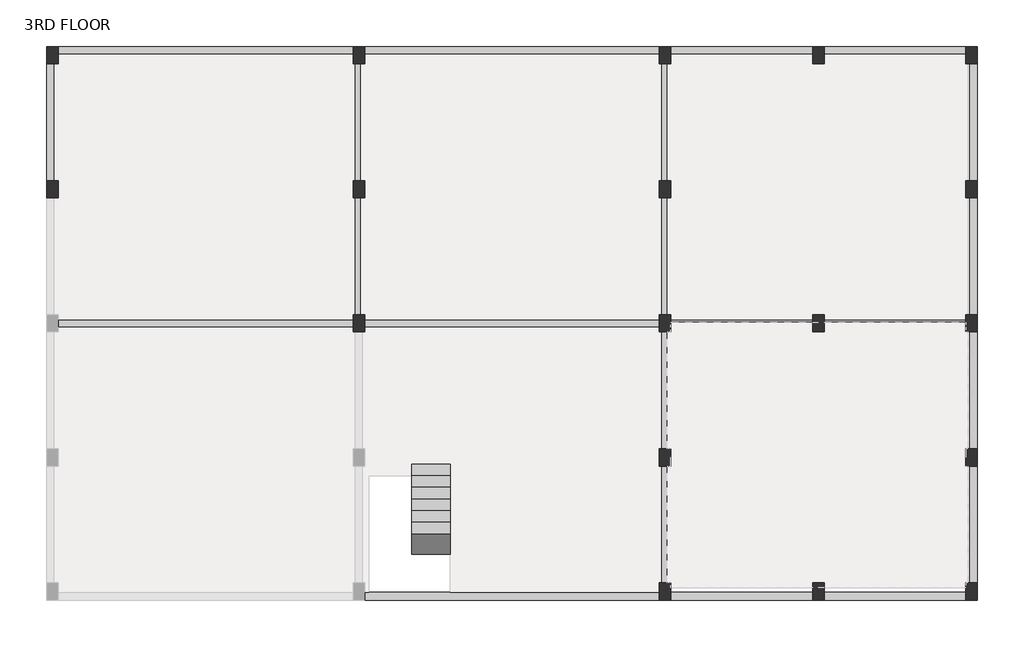
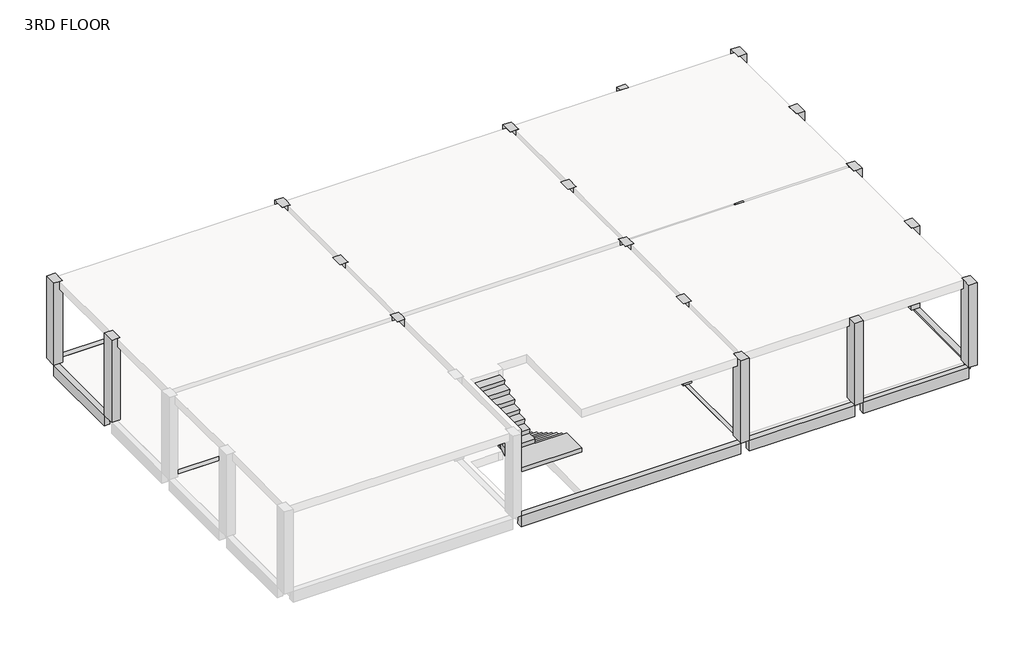
# One storey, part 2 of 2: 22 beams, 18 columns, 1 stair flight.
"""IFC4 building model written with IfcOpenShell, lengths in millimetres."""

from ifc_helpers import new_model, si_unit, frame, origin, place, context, project, spatial, polyline, outline, extrude, faceted_brep, element, save

model = new_model("IFC4")

# Units and contexts
model_context = context("Model", 3, world=origin())
ifc_project = project(units=[si_unit("LENGTHUNIT", "METRE", prefix="MILLI")], contexts=[model_context])

# Site, building, storey
site = spatial("IfcSite", under=ifc_project)
building = spatial("IfcBuilding", under=site)
storey = spatial("IfcBuildingStorey", under=building, Name="3RD FLOOR", Elevation=9144.0)

# Beams
placement = place(None, origin())
element("IfcBeam", 1, ObjectType="M_Concrete-Rectangular Beam : 200MMX400MM", at=placement, inside=storey, context=model_context, shape_type="Brep", body=[
    faceted_brep([(-3980.6874017, 15797.7008557, 9144.0), (-3980.6874017, 15997.7008557, 9144.0), (-11680.6874017, 15997.7008557, 9144.0), (-11680.6874017, 15797.7008557, 9144.0), (-3980.6874017, 15797.7008557, 8744.0), (-3980.6874017, 15797.7008557, 8844.0), (-11680.6874017, 15797.7008557, 8844.0), (-11680.6874017, 15797.7008557, 8744.0), (-3980.6874017, 15997.7008557, 8744.0), (-11680.6874017, 15997.7008557, 8744.0)], [[[0, 1, 2, 3]], [[4, 5, 0, 3, 6, 7]], [[8, 4, 7, 9]], [[1, 8, 9, 2]], [[2, 9, 7, 6, 3]], [[1, 0, 5, 4, 8]]]),
])
element("IfcBeam", 2, ObjectType="M_Concrete-Rectangular Beam : 200MMX400MM", at=placement, inside=storey, context=model_context, shape_type="Brep", body=[
    faceted_brep([(4019.3125983, 15797.7008557, 9144.0), (4019.3125983, 15997.7008557, 9144.0), (-3680.6874017, 15997.7008557, 9144.0), (-3680.6874017, 15797.7008557, 9144.0), (4019.3125983, 15797.7008557, 8744.0), (4019.3125983, 15797.7008557, 8844.0), (-3680.6874017, 15797.7008557, 8844.0), (-3680.6874017, 15797.7008557, 8744.0), (4019.3125983, 15997.7008557, 8744.0), (-3680.6874017, 15997.7008557, 8744.0)], [[[0, 1, 2, 3]], [[4, 5, 0, 3, 6, 7]], [[8, 4, 7, 9]], [[1, 8, 9, 2]], [[1, 0, 5, 4, 8]], [[2, 9, 7, 6, 3]]]),
])
element("IfcBeam", 3, ObjectType="M_Concrete-Rectangular Beam : 200MMX400MM", at=placement, inside=storey, context=model_context, shape_type="Brep", body=[
    faceted_brep([(8019.3125983, 15797.7008557, 9144.0), (8019.3125983, 15997.7008557, 9144.0), (4319.3125983, 15997.7008557, 9144.0), (4319.3125983, 15797.7008557, 9144.0), (8019.3125983, 15797.7008557, 8744.0), (4319.3125983, 15797.7008557, 8844.0), (4319.3125983, 15797.7008557, 8744.0), (8019.3125983, 15997.7008557, 8744.0), (4319.3125983, 15997.7008557, 8744.0)], [[[0, 1, 2, 3]], [[4, 0, 3, 5, 6]], [[7, 4, 6, 8]], [[1, 7, 8, 2]], [[2, 8, 6, 5, 3]], [[1, 0, 4, 7]]]),
])
element("IfcBeam", 4, ObjectType="M_Concrete-Rectangular Beam : 200MMX400MM", at=placement, inside=storey, context=model_context, shape_type="Brep", body=[
    faceted_brep([(12019.3125983, 15797.7008557, 9144.0), (12019.3125983, 15997.7008557, 9144.0), (8319.3125983, 15997.7008557, 9144.0), (8319.3125983, 15797.7008557, 9144.0), (12019.3125983, 15797.7008557, 8744.0), (12019.3125983, 15797.7008557, 8844.0), (8319.3125983, 15797.7008557, 8744.0), (12019.3125983, 15997.7008557, 8744.0), (8319.3125983, 15997.7008557, 8744.0)], [[[0, 1, 2, 3]], [[4, 5, 0, 3, 6]], [[7, 4, 6, 8]], [[1, 7, 8, 2]], [[2, 8, 6, 3]], [[1, 0, 5, 4, 7]]]),
])
element("IfcBeam", 5, ObjectType="M_Concrete-Rectangular Beam : 200MMX400MM", at=placement, inside=storey, context=model_context, shape_type="SweptSolid", body=[
    extrude(outline(polyline([(12319.3125983, 12497.7008557), (12119.3125983, 12497.7008557), (12119.3125983, 15547.7008557), (12319.3125983, 15547.7008557), (12319.3125983, 12497.7008557)])), frame((0.0, 0.0, 8744.0), z_axis=(0.0, 0.0, 1.0), x_axis=(1.0, 0.0, 0.0)), (0.0, 0.0, 1.0), 400.0),
])
element("IfcBeam", 6, ObjectType="M_Concrete-Rectangular Beam : 200MMX400MM", at=placement, inside=storey, context=model_context, shape_type="SweptSolid", body=[
    extrude(outline(polyline([(12319.3125983, 1997.7008557), (12119.3125983, 1997.7008557), (12119.3125983, 5047.7008557), (12319.3125983, 5047.7008557), (12319.3125983, 1997.7008557)])), frame((0.0, 0.0, 8744.0), z_axis=(0.0, 0.0, 1.0), x_axis=(1.0, 0.0, 0.0)), (0.0, 0.0, 1.0), 400.0),
])
element("IfcBeam", 7, ObjectType="M_Concrete-Rectangular Beam : 200MMX400MM", at=placement, inside=storey, context=model_context, shape_type="SweptSolid", body=[
    extrude(outline(polyline([(8319.3125983, 1547.7008557), (8319.3125983, 1747.7008557), (12019.3125983, 1747.7008557), (12019.3125983, 1547.7008557), (8319.3125983, 1547.7008557)])), frame((0.0, 0.0, 8744.0), z_axis=(0.0, 0.0, 1.0), x_axis=(1.0, 0.0, 0.0)), (0.0, 0.0, 1.0), 400.0),
])
element("IfcBeam", 8, ObjectType="M_Concrete-Rectangular Beam : 200MMX400MM", at=placement, inside=storey, context=model_context, shape_type="SweptSolid", body=[
    extrude(outline(polyline([(8019.3125983, 1747.7008557), (8019.3125983, 1547.7008557), (4319.3125983, 1547.7008557), (4319.3125983, 1747.7008557), (8019.3125983, 1747.7008557)])), frame((0.0, 0.0, 8744.0), z_axis=(0.0, 0.0, 1.0), x_axis=(1.0, 0.0, 0.0)), (0.0, 0.0, 1.0), 400.0),
])
element("IfcBeam", 9, ObjectType="M_Concrete-Rectangular Beam : 200MMX400MM", at=placement, inside=storey, context=model_context, shape_type="Brep", body=[
    faceted_brep([(-3680.6874017, 1747.7008557, 9144.0), (-3680.6874017, 1547.7008557, 9144.0), (4019.3125983, 1547.7008557, 9144.0), (4019.3125983, 1747.7008557, 9144.0), (-1437.0874017, 1747.7008557, 9144.0), (-3570.6874017, 1747.7008557, 9144.0), (-3680.6874017, 1747.7008557, 8744.0), (-3680.6874017, 1747.7008557, 8844.0), (4019.3125983, 1747.7008557, 8844.0), (4019.3125983, 1747.7008557, 8744.0), (-3680.6874017, 1547.7008557, 8744.0), (4019.3125983, 1547.7008557, 8744.0)], [[[0, 1, 2, 3, 4, 5]], [[6, 7, 0, 5, 4, 3, 8, 9]], [[10, 6, 9, 11]], [[1, 10, 11, 2]], [[1, 0, 7, 6, 10]], [[2, 11, 9, 8, 3]]]),
])
element("IfcBeam", 10, ObjectType="M_Concrete-Rectangular Beam : 200MMX400MM", at=placement, inside=storey, context=model_context, shape_type="Brep", body=[
    faceted_brep([(-3980.6874017, 8872.7008557, 9144.0), (-11680.6874017, 8872.7008557, 9144.0), (-11680.6874017, 8672.7008557, 9144.0), (-3980.6874017, 8672.7008557, 9144.0), (-11680.6874017, 8672.7008557, 8844.0), (-11680.6874017, 8672.7008557, 8744.0), (-3980.6874017, 8672.7008557, 8744.0), (-3980.6874017, 8672.7008557, 8844.0), (-11680.6874017, 8872.7008557, 8744.0), (-3980.6874017, 8872.7008557, 8744.0), (-3980.6874017, 8872.7008557, 8844.0), (-11680.6874017, 8872.7008557, 8844.0)], [[[0, 1, 2, 3]], [[3, 2, 4, 5, 6, 7]], [[6, 5, 8, 9]], [[1, 0, 10, 9, 8, 11]], [[8, 5, 4, 2, 1, 11]], [[0, 3, 7, 6, 9, 10]]]),
])
element("IfcBeam", 11, ObjectType="M_Concrete-Rectangular Beam : 200MMX400MM", at=placement, inside=storey, context=model_context, shape_type="Brep", body=[
    faceted_brep([(4019.3125983, 8872.7008557, 9144.0), (-3680.6874017, 8872.7008557, 9144.0), (-3680.6874017, 8672.7008557, 9144.0), (4019.3125983, 8672.7008557, 9144.0), (-3680.6874017, 8672.7008557, 8844.0), (-3680.6874017, 8672.7008557, 8744.0), (4019.3125983, 8672.7008557, 8744.0), (4019.3125983, 8672.7008557, 8844.0), (-3680.6874017, 8872.7008557, 8744.0), (4019.3125983, 8872.7008557, 8744.0), (4019.3125983, 8872.7008557, 8844.0), (-3680.6874017, 8872.7008557, 8844.0)], [[[0, 1, 2, 3]], [[3, 2, 4, 5, 6, 7]], [[6, 5, 8, 9]], [[1, 0, 10, 9, 8, 11]], [[8, 5, 4, 2, 1, 11]], [[0, 3, 7, 6, 9, 10]]]),
])
element("IfcBeam", 12, ObjectType="M_Concrete-Rectangular Beam : 200MMX400MM", at=placement, inside=storey, context=model_context, shape_type="Brep", body=[
    faceted_brep([(8019.3125983, 8872.7008557, 9144.0), (4319.3125983, 8872.7008557, 9144.0), (4319.3125983, 8797.7008557, 9144.0), (8019.3125983, 8797.7008557, 9144.0), (4319.3125983, 8672.7008557, 8744.0), (8019.3125983, 8672.7008557, 8744.0), (8019.3125983, 8672.7008557, 8844.0), (4319.3125983, 8672.7008557, 8844.0), (4319.3125983, 8872.7008557, 8744.0), (8019.3125983, 8872.7008557, 8744.0), (8019.3125983, 8872.7008557, 8844.0), (4319.3125983, 8872.7008557, 8844.0), (4319.3125983, 8797.7008557, 8844.0), (8019.3125983, 8797.7008557, 8844.0)], [[[0, 1, 2, 3]], [[4, 5, 6, 7]], [[5, 4, 8, 9]], [[1, 0, 10, 9, 8, 11]], [[8, 4, 7, 12, 2, 1, 11]], [[5, 9, 10, 0, 3, 13, 6]], [[13, 12, 7, 6]], [[12, 13, 3, 2]]]),
])
element("IfcBeam", 13, ObjectType="M_Concrete-Rectangular Beam : 200MMX400MM", at=placement, inside=storey, context=model_context, shape_type="Brep", body=[
    faceted_brep([(-11980.6874017, 12497.7008557, 9144.0), (-11780.6874017, 12497.7008557, 9144.0), (-11780.6874017, 15547.7008557, 9144.0), (-11980.6874017, 15547.7008557, 9144.0), (-11980.6874017, 12497.7008557, 8744.0), (-11980.6874017, 15547.7008557, 8744.0), (-11780.6874017, 12497.7008557, 8744.0), (-11780.6874017, 15547.7008557, 8744.0), (-11780.6874017, 12497.7008557, 8844.0), (-11780.6874017, 15547.7008557, 8844.0)], [[[0, 1, 2, 3]], [[4, 0, 3, 5]], [[6, 4, 5, 7]], [[1, 8, 6, 7, 9, 2]], [[2, 9, 7, 5, 3]], [[1, 0, 4, 6, 8]]]),
])
element("IfcBeam", 14, ObjectType="M_Concrete-Rectangular Beam : 200MMX400MM", at=placement, inside=storey, context=model_context, shape_type="Brep", body=[
    faceted_brep([(12019.3125983, 8872.7008557, 9144.0), (8319.3125983, 8872.7008557, 9144.0), (8319.3125983, 8797.7008557, 9144.0), (12019.3125983, 8797.7008557, 9144.0), (8319.3125983, 8672.7008557, 8744.0), (12019.3125983, 8672.7008557, 8744.0), (12019.3125983, 8672.7008557, 8844.0), (8319.3125983, 8672.7008557, 8844.0), (8319.3125983, 8872.7008557, 8744.0), (12019.3125983, 8872.7008557, 8744.0), (12019.3125983, 8872.7008557, 8844.0), (8319.3125983, 8872.7008557, 8844.0), (12019.3125983, 8797.7008557, 8844.0), (8319.3125983, 8797.7008557, 8844.0)], [[[0, 1, 2, 3]], [[4, 5, 6, 7]], [[5, 4, 8, 9]], [[1, 0, 10, 9, 8, 11]], [[5, 9, 10, 0, 3, 12, 6]], [[8, 4, 7, 13, 2, 1, 11]], [[12, 13, 7, 6]], [[13, 12, 3, 2]]]),
])
element("IfcBeam", 15, ObjectType="M_Concrete-Rectangular Beam : 200MMX400MM", at=placement, inside=storey, context=model_context, shape_type="SweptSolid", body=[
    extrude(outline(polyline([(12319.3125983, 5497.7008557), (12119.3125983, 5497.7008557), (12119.3125983, 8547.7008557), (12319.3125983, 8547.7008557), (12319.3125983, 5497.7008557)])), frame((0.0, 0.0, 8744.0), z_axis=(0.0, 0.0, 1.0), x_axis=(1.0, 0.0, 0.0)), (0.0, 0.0, 1.0), 400.0),
])
element("IfcBeam", 16, ObjectType="M_Concrete-Rectangular Beam : 200MMX400MM", at=placement, inside=storey, context=model_context, shape_type="SweptSolid", body=[
    extrude(outline(polyline([(12119.3125983, 12047.7008557), (12319.3125983, 12047.7008557), (12319.3125983, 8997.7008557), (12119.3125983, 8997.7008557), (12119.3125983, 12047.7008557)])), frame((0.0, 0.0, 8744.0), z_axis=(0.0, 0.0, 1.0), x_axis=(1.0, 0.0, 0.0)), (0.0, 0.0, 1.0), 400.0),
])
element("IfcBeam", 17, ObjectType="M_Concrete-Rectangular Beam : 200MMX400MM", at=placement, inside=storey, context=model_context, shape_type="Brep", body=[
    faceted_brep([(4069.3125983, 5047.7008557, 9144.0), (4069.3125983, 1997.7008557, 9144.0), (4219.3125983, 1997.7008557, 9144.0), (4219.3125983, 5047.7008557, 9144.0), (4269.3125983, 1997.7008557, 8744.0), (4269.3125983, 5047.7008557, 8744.0), (4269.3125983, 5047.7008557, 8844.0), (4269.3125983, 1997.7008557, 8844.0), (4069.3125983, 1997.7008557, 8744.0), (4069.3125983, 5047.7008557, 8744.0), (4069.3125983, 5047.7008557, 8844.0), (4069.3125983, 1997.7008557, 8844.0), (4219.3125983, 1997.7008557, 8844.0), (4219.3125983, 5047.7008557, 8844.0)], [[[0, 1, 2, 3]], [[4, 5, 6, 7]], [[5, 4, 8, 9]], [[1, 0, 10, 9, 8, 11]], [[8, 4, 7, 12, 2, 1, 11]], [[5, 9, 10, 0, 3, 13, 6]], [[13, 12, 7, 6]], [[12, 13, 3, 2]]]),
])
element("IfcBeam", 18, ObjectType="M_Concrete-Rectangular Beam : 200MMX400MM", at=placement, inside=storey, context=model_context, shape_type="Brep", body=[
    faceted_brep([(4069.3125983, 8547.7008557, 9144.0), (4069.3125983, 5497.7008557, 9144.0), (4219.3125983, 5497.7008557, 9144.0), (4219.3125983, 8547.7008557, 9144.0), (4269.3125983, 5497.7008557, 8744.0), (4269.3125983, 8547.7008557, 8744.0), (4269.3125983, 8547.7008557, 8844.0), (4269.3125983, 5497.7008557, 8844.0), (4069.3125983, 5497.7008557, 8744.0), (4069.3125983, 8547.7008557, 8744.0), (4069.3125983, 8547.7008557, 8844.0), (4069.3125983, 5497.7008557, 8844.0), (4219.3125983, 8547.7008557, 8844.0), (4219.3125983, 5497.7008557, 8844.0)], [[[0, 1, 2, 3]], [[4, 5, 6, 7]], [[5, 4, 8, 9]], [[1, 0, 10, 9, 8, 11]], [[5, 9, 10, 0, 3, 12, 6]], [[8, 4, 7, 13, 2, 1, 11]], [[12, 13, 7, 6]], [[13, 12, 3, 2]]]),
])
element("IfcBeam", 19, ObjectType="M_Concrete-Rectangular Beam : 200MMX400MM", at=placement, inside=storey, context=model_context, shape_type="Brep", body=[
    faceted_brep([(4069.3125983, 12047.7008557, 9144.0), (4069.3125983, 8997.7008557, 9144.0), (4219.3125983, 8997.7008557, 9144.0), (4219.3125983, 12047.7008557, 9144.0), (4269.3125983, 8997.7008557, 8744.0), (4269.3125983, 12047.7008557, 8744.0), (4269.3125983, 12047.7008557, 8844.0), (4269.3125983, 8997.7008557, 8844.0), (4069.3125983, 8997.7008557, 8744.0), (4069.3125983, 12047.7008557, 8744.0), (4069.3125983, 12047.7008557, 8844.0), (4069.3125983, 8997.7008557, 8844.0), (4219.3125983, 8997.7008557, 8844.0), (4219.3125983, 12047.7008557, 8844.0)], [[[0, 1, 2, 3]], [[4, 5, 6, 7]], [[5, 4, 8, 9]], [[1, 0, 10, 9, 8, 11]], [[8, 4, 7, 12, 2, 1, 11]], [[5, 9, 10, 0, 3, 13, 6]], [[13, 12, 7, 6]], [[12, 13, 3, 2]]]),
])
element("IfcBeam", 20, ObjectType="M_Concrete-Rectangular Beam : 200MMX400MM", at=placement, inside=storey, context=model_context, shape_type="Brep", body=[
    faceted_brep([(4069.3125983, 15547.7008557, 9144.0), (4069.3125983, 12497.7008557, 9144.0), (4219.3125983, 12497.7008557, 9144.0), (4219.3125983, 15547.7008557, 9144.0), (4269.3125983, 12497.7008557, 8744.0), (4269.3125983, 15547.7008557, 8744.0), (4269.3125983, 15547.7008557, 8844.0), (4269.3125983, 12497.7008557, 8844.0), (4069.3125983, 12497.7008557, 8744.0), (4069.3125983, 15547.7008557, 8744.0), (4069.3125983, 15547.7008557, 8844.0), (4069.3125983, 12497.7008557, 8844.0), (4219.3125983, 15547.7008557, 8844.0), (4219.3125983, 12497.7008557, 8844.0)], [[[0, 1, 2, 3]], [[4, 5, 6, 7]], [[5, 4, 8, 9]], [[1, 0, 10, 9, 8, 11]], [[5, 9, 10, 0, 3, 12, 6]], [[8, 4, 7, 13, 2, 1, 11]], [[12, 13, 7, 6]], [[13, 12, 3, 2]]]),
])
element("IfcBeam", 21, ObjectType="M_Concrete-Rectangular Beam : 200MMX400MM", at=placement, inside=storey, context=model_context, shape_type="Brep", body=[
    faceted_brep([(-3930.6874017, 12047.7008557, 9144.0), (-3930.6874017, 8997.7008557, 9144.0), (-3780.6874017, 8997.7008557, 9144.0), (-3780.6874017, 12047.7008557, 9144.0), (-3730.6874017, 8997.7008557, 8744.0), (-3730.6874017, 12047.7008557, 8744.0), (-3730.6874017, 12047.7008557, 8844.0), (-3730.6874017, 8997.7008557, 8844.0), (-3930.6874017, 8997.7008557, 8744.0), (-3930.6874017, 12047.7008557, 8744.0), (-3930.6874017, 12047.7008557, 8844.0), (-3930.6874017, 8997.7008557, 8844.0), (-3780.6874017, 12047.7008557, 8844.0), (-3780.6874017, 8997.7008557, 8844.0)], [[[0, 1, 2, 3]], [[4, 5, 6, 7]], [[5, 4, 8, 9]], [[1, 0, 10, 9, 8, 11]], [[5, 9, 10, 0, 3, 12, 6]], [[8, 4, 7, 13, 2, 1, 11]], [[12, 13, 7, 6]], [[13, 12, 3, 2]]]),
])
element("IfcBeam", 22, ObjectType="M_Concrete-Rectangular Beam : 200MMX400MM", at=placement, inside=storey, context=model_context, shape_type="Brep", body=[
    faceted_brep([(-3930.6874017, 15547.7008557, 9144.0), (-3930.6874017, 12497.7008557, 9144.0), (-3780.6874017, 12497.7008557, 9144.0), (-3780.6874017, 15547.7008557, 9144.0), (-3730.6874017, 12497.7008557, 8744.0), (-3730.6874017, 15547.7008557, 8744.0), (-3730.6874017, 15547.7008557, 8844.0), (-3730.6874017, 12497.7008557, 8844.0), (-3930.6874017, 12497.7008557, 8744.0), (-3930.6874017, 15547.7008557, 8744.0), (-3930.6874017, 15547.7008557, 8844.0), (-3930.6874017, 12497.7008557, 8844.0), (-3780.6874017, 15547.7008557, 8844.0), (-3780.6874017, 12497.7008557, 8844.0)], [[[0, 1, 2, 3]], [[4, 5, 6, 7]], [[5, 4, 8, 9]], [[1, 0, 10, 9, 8, 11]], [[5, 9, 10, 0, 3, 12, 6]], [[8, 4, 7, 13, 2, 1, 11]], [[12, 13, 7, 6]], [[13, 12, 3, 2]]]),
])

# Columns
element("IfcColumn", 23, ObjectType="M_Concrete-Rectangular-Column : 300 x 450mm", at=placement, inside=storey, context=model_context, shape_type="Brep", body=[
    faceted_brep([(-11680.6874017, 15997.7008557, 9144.0), (-11680.6874017, 15547.7008557, 9144.0), (-11980.6874017, 15547.7008557, 9144.0), (-11980.6874017, 15997.7008557, 9144.0), (-11680.6874017, 15997.7008557, 12192.0), (-11680.6874017, 15797.7008557, 12192.0), (-11680.6874017, 15547.7008557, 12192.0), (-11680.6874017, 15547.7008557, 11892.0), (-11780.6874017, 15547.7008557, 12192.0), (-11980.6874017, 15547.7008557, 12192.0), (-11980.6874017, 15997.7008557, 12192.0)], [[[0, 1, 2, 3]], [[1, 0, 4, 5, 6, 7]], [[2, 1, 7, 6, 8, 9]], [[3, 2, 9, 10]], [[0, 3, 10, 4]], [[10, 9, 8, 6, 5, 4]]]),
])
element("IfcColumn", 24, ObjectType="M_Concrete-Rectangular-Column : 300 x 450mm", at=placement, inside=storey, context=model_context, shape_type="Brep", body=[
    faceted_brep([(-3680.6874017, 15997.7008557, 9144.0), (-3680.6874017, 15547.7008557, 9144.0), (-3980.6874017, 15547.7008557, 9144.0), (-3980.6874017, 15997.7008557, 9144.0), (-3680.6874017, 15997.7008557, 12192.0), (-3680.6874017, 15797.7008557, 12192.0), (-3680.6874017, 15547.7008557, 12192.0), (-3680.6874017, 15547.7008557, 11892.0), (-3780.6874017, 15547.7008557, 12192.0), (-3930.6874017, 15547.7008557, 12192.0), (-3980.6874017, 15547.7008557, 12192.0), (-3980.6874017, 15547.7008557, 11892.0), (-3980.6874017, 15797.7008557, 12192.0), (-3980.6874017, 15997.7008557, 12192.0)], [[[0, 1, 2, 3]], [[1, 0, 4, 5, 6, 7]], [[2, 1, 7, 6, 8, 9, 10, 11]], [[3, 2, 11, 10, 12, 13]], [[0, 3, 13, 4]], [[4, 13, 12, 10, 9, 8, 6, 5]]]),
])
element("IfcColumn", 25, ObjectType="M_Concrete-Rectangular-Column : 300 x 450mm", at=placement, inside=storey, context=model_context, shape_type="Brep", body=[
    faceted_brep([(-3680.6874017, 12497.7008557, 9144.0), (-3680.6874017, 12047.7008557, 9144.0), (-3980.6874017, 12047.7008557, 9144.0), (-3980.6874017, 12497.7008557, 9144.0), (-3680.6874017, 12497.7008557, 11892.0), (-3680.6874017, 12497.7008557, 12192.0), (-3680.6874017, 12047.7008557, 12192.0), (-3680.6874017, 12047.7008557, 11892.0), (-3780.6874017, 12047.7008557, 12192.0), (-3930.6874017, 12047.7008557, 12192.0), (-3980.6874017, 12047.7008557, 12192.0), (-3980.6874017, 12047.7008557, 11892.0), (-3980.6874017, 12497.7008557, 12192.0), (-3980.6874017, 12497.7008557, 11892.0), (-3930.6874017, 12497.7008557, 12192.0), (-3780.6874017, 12497.7008557, 12192.0)], [[[0, 1, 2, 3]], [[1, 0, 4, 5, 6, 7]], [[2, 1, 7, 6, 8, 9, 10, 11]], [[3, 2, 11, 10, 12, 13]], [[0, 3, 13, 12, 14, 15, 5, 4]], [[6, 5, 15, 14, 12, 10, 9, 8]]]),
])
element("IfcColumn", 26, ObjectType="M_Concrete-Rectangular-Column : 300 x 450mm", at=placement, inside=storey, context=model_context, shape_type="Brep", body=[
    faceted_brep([(-3680.6874017, 8997.7008557, 9144.0), (-3680.6874017, 8547.7008557, 9144.0), (-3980.6874017, 8547.7008557, 9144.0), (-3980.6874017, 8997.7008557, 9144.0), (-3680.6874017, 8997.7008557, 11892.0), (-3680.6874017, 8997.7008557, 12192.0), (-3680.6874017, 8872.7008557, 12192.0), (-3680.6874017, 8672.7008557, 12192.0), (-3680.6874017, 8547.7008557, 12192.0), (-3680.6874017, 8547.7008557, 11892.0), (-3730.6874017, 8547.7008557, 12192.0), (-3930.6874017, 8547.7008557, 12192.0), (-3980.6874017, 8547.7008557, 12192.0), (-3980.6874017, 8547.7008557, 11892.0), (-3980.6874017, 8672.7008557, 12192.0), (-3980.6874017, 8872.7008557, 12192.0), (-3980.6874017, 8997.7008557, 12192.0), (-3980.6874017, 8997.7008557, 11892.0), (-3930.6874017, 8997.7008557, 12192.0), (-3780.6874017, 8997.7008557, 12192.0)], [[[0, 1, 2, 3]], [[1, 0, 4, 5, 6, 7, 8, 9]], [[2, 1, 9, 8, 10, 11, 12, 13]], [[3, 2, 13, 12, 14, 15, 16, 17]], [[0, 3, 17, 16, 18, 19, 5, 4]], [[18, 16, 15, 14, 12, 11, 10, 8, 7, 6, 5, 19]]]),
])
element("IfcColumn", 27, ObjectType="M_Concrete-Rectangular-Column : 300 x 450mm", at=placement, inside=storey, context=model_context, shape_type="Brep", body=[
    faceted_brep([(4319.3125983, 15997.7008557, 9144.0), (4319.3125983, 15547.7008557, 9144.0), (4019.3125983, 15547.7008557, 9144.0), (4019.3125983, 15997.7008557, 9144.0), (4319.3125983, 15997.7008557, 12192.0), (4319.3125983, 15797.7008557, 12192.0), (4319.3125983, 15547.7008557, 12192.0), (4319.3125983, 15547.7008557, 11892.0), (4219.3125983, 15547.7008557, 12192.0), (4069.3125983, 15547.7008557, 12192.0), (4019.3125983, 15547.7008557, 12192.0), (4019.3125983, 15547.7008557, 11892.0), (4019.3125983, 15797.7008557, 12192.0), (4019.3125983, 15997.7008557, 12192.0)], [[[0, 1, 2, 3]], [[1, 0, 4, 5, 6, 7]], [[2, 1, 7, 6, 8, 9, 10, 11]], [[3, 2, 11, 10, 12, 13]], [[0, 3, 13, 4]], [[4, 13, 12, 10, 9, 8, 6, 5]]]),
])
element("IfcColumn", 28, ObjectType="M_Concrete-Rectangular-Column : 300 x 450mm", at=placement, inside=storey, context=model_context, shape_type="Brep", body=[
    faceted_brep([(4319.3125983, 8997.7008557, 9144.0), (4319.3125983, 8547.7008557, 9144.0), (4019.3125983, 8547.7008557, 9144.0), (4019.3125983, 8997.7008557, 9144.0), (4319.3125983, 8997.7008557, 11892.0), (4319.3125983, 8997.7008557, 12192.0), (4319.3125983, 8872.7008557, 12192.0), (4319.3125983, 8797.7008557, 12192.0), (4319.3125983, 8547.7008557, 12192.0), (4319.3125983, 8547.7008557, 11892.0), (4219.3125983, 8547.7008557, 12192.0), (4069.3125983, 8547.7008557, 12192.0), (4019.3125983, 8547.7008557, 12192.0), (4019.3125983, 8547.7008557, 11892.0), (4019.3125983, 8672.7008557, 12192.0), (4019.3125983, 8872.7008557, 12192.0), (4019.3125983, 8997.7008557, 12192.0), (4019.3125983, 8997.7008557, 11892.0), (4069.3125983, 8997.7008557, 12192.0), (4219.3125983, 8997.7008557, 12192.0)], [[[0, 1, 2, 3]], [[1, 0, 4, 5, 6, 7, 8, 9]], [[2, 1, 9, 8, 10, 11, 12, 13]], [[3, 2, 13, 12, 14, 15, 16, 17]], [[0, 3, 17, 16, 18, 19, 5, 4]], [[18, 16, 15, 14, 12, 11, 10, 8, 7, 6, 5, 19]]]),
])
element("IfcColumn", 29, ObjectType="M_Concrete-Rectangular-Column : 300 x 450mm", at=placement, inside=storey, context=model_context, shape_type="Brep", body=[
    faceted_brep([(4319.3125983, 1997.7008557, 9144.0), (4319.3125983, 1547.7008557, 9144.0), (4019.3125983, 1547.7008557, 9144.0), (4019.3125983, 1997.7008557, 9144.0), (4319.3125983, 1997.7008557, 11892.0), (4319.3125983, 1997.7008557, 12192.0), (4319.3125983, 1872.7008557, 12192.0), (4319.3125983, 1547.7008557, 12192.0), (4019.3125983, 1547.7008557, 12192.0), (4019.3125983, 1747.7008557, 12192.0), (4019.3125983, 1997.7008557, 12192.0), (4019.3125983, 1997.7008557, 11892.0), (4069.3125983, 1997.7008557, 12192.0), (4219.3125983, 1997.7008557, 12192.0)], [[[0, 1, 2, 3]], [[1, 0, 4, 5, 6, 7]], [[2, 1, 7, 8]], [[3, 2, 8, 9, 10, 11]], [[0, 3, 11, 10, 12, 13, 5, 4]], [[8, 7, 6, 5, 13, 12, 10, 9]]]),
])
element("IfcColumn", 30, ObjectType="M_Concrete-Rectangular-Column : 300 x 450mm", at=placement, inside=storey, context=model_context, shape_type="SweptSolid", body=[
    extrude(outline(polyline([(15997.7008557, 9144.0), (15547.7008557, 9144.0), (15547.7008557, 11892.0), (15797.7008557, 11892.0), (15797.7008557, 12192.0), (15997.7008557, 12192.0), (15997.7008557, 9144.0)])), frame((8019.3125983, 0.0, 0.0), z_axis=(1.0, 0.0, 0.0), x_axis=(0.0, 1.0, 0.0)), (0.0, 0.0, 1.0), 300.0),
])
element("IfcColumn", 31, ObjectType="M_Concrete-Rectangular-Column : 300 x 450mm", at=placement, inside=storey, context=model_context, shape_type="SweptSolid", body=[
    extrude(outline(polyline([(1997.7008557, 9144.0), (1547.7008557, 9144.0), (1547.7008557, 12192.0), (1872.7008557, 12192.0), (1872.7008557, 11892.0), (1997.7008557, 11892.0), (1997.7008557, 9144.0)])), frame((8019.3125983, 0.0, 0.0), z_axis=(1.0, 0.0, 0.0), x_axis=(0.0, 1.0, 0.0)), (0.0, 0.0, 1.0), 300.0),
])
element("IfcColumn", 32, ObjectType="M_Concrete-Rectangular-Column : 300 x 450mm", at=placement, inside=storey, context=model_context, shape_type="Brep", body=[
    faceted_brep([(12319.3125983, 12497.7008557, 9144.0), (12319.3125983, 12047.7008557, 9144.0), (12019.3125983, 12047.7008557, 9144.0), (12019.3125983, 12497.7008557, 9144.0), (12319.3125983, 12497.7008557, 12192.0), (12319.3125983, 12047.7008557, 12192.0), (12069.3125983, 12047.7008557, 12192.0), (12019.3125983, 12047.7008557, 12192.0), (12019.3125983, 12047.7008557, 11892.0), (12019.3125983, 12497.7008557, 12192.0), (12019.3125983, 12497.7008557, 11892.0), (12069.3125983, 12497.7008557, 12192.0)], [[[0, 1, 2, 3]], [[1, 0, 4, 5]], [[2, 1, 5, 6, 7, 8]], [[3, 2, 8, 7, 9, 10]], [[0, 3, 10, 9, 11, 4]], [[5, 4, 11, 9, 7, 6]]]),
])
element("IfcColumn", 33, ObjectType="M_Concrete-Rectangular-Column : 300 x 450mm", at=placement, inside=storey, context=model_context, shape_type="Brep", body=[
    faceted_brep([(12319.3125983, 5497.7008557, 9144.0), (12319.3125983, 5047.7008557, 9144.0), (12019.3125983, 5047.7008557, 9144.0), (12019.3125983, 5497.7008557, 9144.0), (12319.3125983, 5497.7008557, 12192.0), (12319.3125983, 5047.7008557, 12192.0), (12069.3125983, 5047.7008557, 12192.0), (12019.3125983, 5047.7008557, 12192.0), (12019.3125983, 5047.7008557, 11892.0), (12019.3125983, 5497.7008557, 12192.0), (12019.3125983, 5497.7008557, 11892.0), (12069.3125983, 5497.7008557, 12192.0)], [[[0, 1, 2, 3]], [[1, 0, 4, 5]], [[2, 1, 5, 6, 7, 8]], [[3, 2, 8, 7, 9, 10]], [[0, 3, 10, 9, 11, 4]], [[5, 4, 11, 9, 7, 6]]]),
])
element("IfcColumn", 34, ObjectType="M_Concrete-Rectangular-Column : 300 x 450mm", at=placement, inside=storey, context=model_context, shape_type="Brep", body=[
    faceted_brep([(12319.3125983, 15997.7008557, 9144.0), (12319.3125983, 15547.7008557, 9144.0), (12019.3125983, 15547.7008557, 9144.0), (12019.3125983, 15997.7008557, 9144.0), (12319.3125983, 15997.7008557, 12192.0), (12319.3125983, 15547.7008557, 12192.0), (12069.3125983, 15547.7008557, 12192.0), (12019.3125983, 15547.7008557, 12192.0), (12019.3125983, 15547.7008557, 11892.0), (12019.3125983, 15797.7008557, 12192.0), (12019.3125983, 15997.7008557, 12192.0)], [[[0, 1, 2, 3]], [[1, 0, 4, 5]], [[2, 1, 5, 6, 7, 8]], [[3, 2, 8, 7, 9, 10]], [[0, 3, 10, 4]], [[5, 4, 10, 9, 7, 6]]]),
])
element("IfcColumn", 35, ObjectType="M_Concrete-Rectangular-Column : 300 x 450mm", at=placement, inside=storey, context=model_context, shape_type="Brep", body=[
    faceted_brep([(12319.3125983, 1997.7008557, 9144.0), (12319.3125983, 1547.7008557, 9144.0), (12019.3125983, 1547.7008557, 9144.0), (12019.3125983, 1997.7008557, 9144.0), (12319.3125983, 1997.7008557, 12192.0), (12319.3125983, 1547.7008557, 12192.0), (12019.3125983, 1547.7008557, 12192.0), (12019.3125983, 1872.7008557, 12192.0), (12019.3125983, 1997.7008557, 12192.0), (12019.3125983, 1997.7008557, 11892.0), (12069.3125983, 1997.7008557, 12192.0)], [[[0, 1, 2, 3]], [[1, 0, 4, 5]], [[2, 1, 5, 6]], [[3, 2, 6, 7, 8, 9]], [[0, 3, 9, 8, 10, 4]], [[5, 4, 10, 8, 7, 6]]]),
])
element("IfcColumn", 36, ObjectType="M_Concrete-Rectangular-Column : 300 x 450mm", at=placement, inside=storey, context=model_context, shape_type="Brep", body=[
    faceted_brep([(-11680.6874017, 12497.7008557, 9144.0), (-11680.6874017, 12047.7008557, 9144.0), (-11980.6874017, 12047.7008557, 9144.0), (-11980.6874017, 12497.7008557, 9144.0), (-11680.6874017, 12497.7008557, 11892.0), (-11680.6874017, 12497.7008557, 12192.0), (-11680.6874017, 12047.7008557, 12192.0), (-11680.6874017, 12047.7008557, 11892.0), (-11780.6874017, 12047.7008557, 12192.0), (-11980.6874017, 12047.7008557, 12192.0), (-11980.6874017, 12497.7008557, 12192.0), (-11780.6874017, 12497.7008557, 12192.0)], [[[0, 1, 2, 3]], [[1, 0, 4, 5, 6, 7]], [[2, 1, 7, 6, 8, 9]], [[3, 2, 9, 10]], [[0, 3, 10, 11, 5, 4]], [[6, 5, 11, 10, 9, 8]]]),
])
element("IfcColumn", 37, ObjectType="M_Concrete-Rectangular-Column : 300 x 450mm", at=placement, inside=storey, context=model_context, shape_type="Brep", body=[
    faceted_brep([(12319.3125983, 8997.7008557, 9144.0), (12319.3125983, 8547.7008557, 9144.0), (12019.3125983, 8547.7008557, 9144.0), (12019.3125983, 8997.7008557, 9144.0), (12319.3125983, 8997.7008557, 12192.0), (12319.3125983, 8547.7008557, 12192.0), (12069.3125983, 8547.7008557, 12192.0), (12019.3125983, 8547.7008557, 12192.0), (12019.3125983, 8547.7008557, 11892.0), (12019.3125983, 8797.7008557, 12192.0), (12019.3125983, 8872.7008557, 12192.0), (12019.3125983, 8997.7008557, 12192.0), (12019.3125983, 8997.7008557, 11892.0), (12069.3125983, 8997.7008557, 12192.0)], [[[0, 1, 2, 3]], [[1, 0, 4, 5]], [[2, 1, 5, 6, 7, 8]], [[3, 2, 8, 7, 9, 10, 11, 12]], [[0, 3, 12, 11, 13, 4]], [[5, 4, 13, 11, 10, 9, 7, 6]]]),
])
element("IfcColumn", 38, ObjectType="M_Concrete-Rectangular-Column : 300 x 450mm", at=placement, inside=storey, context=model_context, shape_type="Brep", body=[
    faceted_brep([(8319.3125983, 8997.7008557, 9144.0), (8319.3125983, 8547.7008557, 9144.0), (8019.3125983, 8547.7008557, 9144.0), (8019.3125983, 8997.7008557, 9144.0), (8319.3125983, 8997.7008557, 11892.0), (8319.3125983, 8872.7008557, 11892.0), (8319.3125983, 8872.7008557, 12192.0), (8319.3125983, 8797.7008557, 12192.0), (8319.3125983, 8797.7008557, 11892.0), (8319.3125983, 8547.7008557, 11892.0), (8019.3125983, 8547.7008557, 11892.0), (8019.3125983, 8672.7008557, 11892.0), (8019.3125983, 8797.7008557, 11892.0), (8019.3125983, 8797.7008557, 12192.0), (8019.3125983, 8872.7008557, 12192.0), (8019.3125983, 8872.7008557, 11892.0), (8019.3125983, 8997.7008557, 11892.0)], [[[0, 1, 2, 3]], [[1, 0, 4, 5, 6, 7, 8, 9]], [[2, 1, 9, 10]], [[3, 2, 10, 11, 12, 13, 14, 15, 16]], [[0, 3, 16, 4]], [[14, 13, 7, 6]], [[8, 12, 11, 10, 9]], [[5, 15, 14, 6]], [[12, 8, 7, 13]], [[15, 5, 4, 16]]]),
])
element("IfcColumn", 39, ObjectType="M_Concrete-Rectangular-Column : 300 x 450mm", at=placement, inside=storey, context=model_context, shape_type="Brep", body=[
    faceted_brep([(4319.3125983, 12497.7008557, 9144.0), (4319.3125983, 12047.7008557, 9144.0), (4019.3125983, 12047.7008557, 9144.0), (4019.3125983, 12497.7008557, 9144.0), (4319.3125983, 12497.7008557, 11892.0), (4319.3125983, 12497.7008557, 12192.0), (4319.3125983, 12047.7008557, 12192.0), (4319.3125983, 12047.7008557, 11892.0), (4219.3125983, 12047.7008557, 12192.0), (4069.3125983, 12047.7008557, 12192.0), (4019.3125983, 12047.7008557, 12192.0), (4019.3125983, 12047.7008557, 11892.0), (4019.3125983, 12497.7008557, 12192.0), (4019.3125983, 12497.7008557, 11892.0), (4069.3125983, 12497.7008557, 12192.0), (4219.3125983, 12497.7008557, 12192.0)], [[[0, 1, 2, 3]], [[1, 0, 4, 5, 6, 7]], [[2, 1, 7, 6, 8, 9, 10, 11]], [[3, 2, 11, 10, 12, 13]], [[0, 3, 13, 12, 14, 15, 5, 4]], [[6, 5, 15, 14, 12, 10, 9, 8]]]),
])
element("IfcColumn", 40, ObjectType="M_Concrete-Rectangular-Column : 300 x 450mm", at=placement, inside=storey, context=model_context, shape_type="Brep", body=[
    faceted_brep([(4319.3125983, 5497.7008557, 9144.0), (4319.3125983, 5047.7008557, 9144.0), (4019.3125983, 5047.7008557, 9144.0), (4019.3125983, 5497.7008557, 9144.0), (4319.3125983, 5497.7008557, 11892.0), (4319.3125983, 5497.7008557, 12192.0), (4319.3125983, 5047.7008557, 12192.0), (4319.3125983, 5047.7008557, 11892.0), (4219.3125983, 5047.7008557, 12192.0), (4069.3125983, 5047.7008557, 12192.0), (4019.3125983, 5047.7008557, 12192.0), (4019.3125983, 5047.7008557, 11892.0), (4019.3125983, 5497.7008557, 12192.0), (4019.3125983, 5497.7008557, 11892.0), (4069.3125983, 5497.7008557, 12192.0), (4219.3125983, 5497.7008557, 12192.0)], [[[0, 1, 2, 3]], [[1, 0, 4, 5, 6, 7]], [[2, 1, 7, 6, 8, 9, 10, 11]], [[3, 2, 11, 10, 12, 13]], [[0, 3, 13, 12, 14, 15, 5, 4]], [[6, 5, 15, 14, 12, 10, 9, 8]]]),
])

# Stair flight
element("IfcStairFlight", 41, ObjectType="25 mm Nosing", at=placement, inside=storey, context=model_context, shape_type="Brep", body=[
    faceted_brep([(-1437.0874017, 5100.5008557, 9323.2941176), (-2453.0874017, 5100.5008557, 9323.2941176), (-2453.0874017, 4770.7008557, 9323.2941176), (-1437.0874017, 4770.7008557, 9323.2941176), (-1437.0874017, 4770.7008557, 9149.2669154), (-1437.0874017, 4779.6546118, 9144.0), (-1437.0874017, 5075.5008557, 9144.0), (-2453.0874017, 5075.5008557, 9144.0), (-2453.0874017, 4779.6546118, 9144.0), (-2453.0874017, 4770.7008557, 9149.2669154), (-1437.0874017, 4795.7008557, 9502.5882353), (-2453.0874017, 4795.7008557, 9502.5882353), (-2453.0874017, 4465.9008557, 9502.5882353), (-1437.0874017, 4465.9008557, 9502.5882353), (-1437.0874017, 4465.9008557, 9328.561033), (-2453.0874017, 4465.9008557, 9328.561033), (-1437.0874017, 4490.9008557, 9681.8823529), (-2453.0874017, 4490.9008557, 9681.8823529), (-2453.0874017, 4161.1008557, 9681.8823529), (-1437.0874017, 4161.1008557, 9681.8823529), (-1437.0874017, 4161.1008557, 9507.8551507), (-2453.0874017, 4161.1008557, 9507.8551507), (-1437.0874017, 4186.1008557, 9861.1764706), (-2453.0874017, 4186.1008557, 9861.1764706), (-2453.0874017, 3856.3008557, 9861.1764706), (-1437.0874017, 3856.3008557, 9861.1764706), (-1437.0874017, 3856.3008557, 9687.1492683), (-2453.0874017, 3856.3008557, 9687.1492683), (-1437.0874017, 3881.3008557, 10040.4705882), (-2453.0874017, 3881.3008557, 10040.4705882), (-2453.0874017, 3551.5008557, 10040.4705882), (-1437.0874017, 3551.5008557, 10040.4705882), (-1437.0874017, 3551.5008557, 9866.443386), (-2453.0874017, 3551.5008557, 9866.443386), (-1437.0874017, 3576.5008557, 10219.7647059), (-2453.0874017, 3576.5008557, 10219.7647059), (-2453.0874017, 3246.7008557, 10219.7647059), (-1437.0874017, 3246.7008557, 10219.7647059), (-1437.0874017, 3246.7008557, 10045.7375036), (-2453.0874017, 3246.7008557, 10045.7375036), (-1437.0874017, 3271.7008557, 10399.0588235), (-2453.0874017, 3271.7008557, 10399.0588235), (-2453.0874017, 2941.9008557, 10399.0588235), (-1437.0874017, 2941.9008557, 10399.0588235), (-1437.0874017, 2941.9008557, 10225.0316213), (-2453.0874017, 2941.9008557, 10225.0316213), (-1437.0874017, 2966.9008557, 10578.3529412), (-2453.0874017, 2966.9008557, 10578.3529412), (-2453.0874017, 2637.1008557, 10578.3529412), (-1437.0874017, 2637.1008557, 10578.3529412), (-1437.0874017, 2637.1008557, 10404.3257389), (-2453.0874017, 2291.4546118, 10607.6470588), (-2453.0874017, 2641.1855014, 10607.6470588), (-3570.6874017, 2687.1008557, 10757.6470588), (-3570.6874017, 1747.7008557, 10757.6470588), (-1437.0874017, 1747.7008557, 10757.6470588), (-1437.0874017, 2291.4546118, 10757.6470588), (-1437.0874017, 2662.1008557, 10757.6470588), (-2453.0874017, 2662.1008557, 10757.6470588), (-2554.6874017, 2662.1008557, 10757.6470588), (-2554.6874017, 2687.1008557, 10757.6470588), (-3570.6874017, 2687.1008557, 10607.6470588), (-3570.6874017, 1747.7008557, 10607.6470588), (-1437.0874017, 1747.7008557, 10607.6470588), (-1437.0874017, 2291.4546118, 10607.6470588), (-2453.0874017, 2662.1008557, 10607.6470588), (-2554.6874017, 2662.1008557, 10607.6470588), (-2554.6874017, 2687.1008557, 10607.6470588), (-3570.6874017, 2662.1008557, 10936.9411765), (-2554.6874017, 2662.1008557, 10936.9411765), (-2554.6874017, 2727.9470995, 10936.9411765), (-2554.6874017, 2991.9008557, 10936.9411765), (-3570.6874017, 2991.9008557, 10936.9411765), (-3570.6874017, 2727.9470995, 10936.9411765), (-3570.6874017, 2991.9008557, 10762.9139742), (-3570.6874017, 2727.9470995, 10607.6470588), (-2554.6874017, 2727.9470995, 10607.6470588), (-2554.6874017, 2991.9008557, 10762.9139742), (-3570.6874017, 2966.9008557, 11116.2352941), (-2554.6874017, 2966.9008557, 11116.2352941), (-2554.6874017, 3296.7008557, 11116.2352941), (-3570.6874017, 3296.7008557, 11116.2352941), (-3570.6874017, 3296.7008557, 10942.2080919), (-2554.6874017, 3296.7008557, 10942.2080919), (-3570.6874017, 3271.7008557, 11295.5294118), (-2554.6874017, 3271.7008557, 11295.5294118), (-2554.6874017, 3601.5008557, 11295.5294118), (-3570.6874017, 3601.5008557, 11295.5294118), (-3570.6874017, 3601.5008557, 11121.5022095), (-2554.6874017, 3601.5008557, 11121.5022095), (-3570.6874017, 3576.5008557, 11474.8235294), (-2554.6874017, 3576.5008557, 11474.8235294), (-2554.6874017, 3906.3008557, 11474.8235294), (-3570.6874017, 3906.3008557, 11474.8235294), (-3570.6874017, 3906.3008557, 11300.7963271), (-2554.6874017, 3906.3008557, 11300.7963271), (-3570.6874017, 3881.3008557, 11654.1176471), (-2554.6874017, 3881.3008557, 11654.1176471), (-2554.6874017, 4211.1008557, 11654.1176471), (-3570.6874017, 4211.1008557, 11654.1176471), (-3570.6874017, 4211.1008557, 11480.0904448), (-2554.6874017, 4211.1008557, 11480.0904448), (-3570.6874017, 4186.1008557, 11833.4117647), (-2554.6874017, 4186.1008557, 11833.4117647), (-2554.6874017, 4515.9008557, 11833.4117647), (-3570.6874017, 4515.9008557, 11833.4117647), (-3570.6874017, 4515.9008557, 11659.3845624), (-2554.6874017, 4515.9008557, 11659.3845624), (-3570.6874017, 4490.9008557, 12012.7058824), (-2554.6874017, 4490.9008557, 12012.7058824), (-2554.6874017, 4795.7008557, 12012.7058824), (-3570.6874017, 4795.7008557, 12012.7058824), (-3570.6874017, 4795.7008557, 11823.9727977), (-2554.6874017, 4795.7008557, 11823.9727977)], [[[0, 1, 2, 3]], [[0, 3, 4, 5, 6]], [[2, 1, 7, 8, 9]], [[10, 11, 12, 13]], [[10, 13, 14, 4, 3]], [[12, 11, 2, 9, 15]], [[16, 17, 18, 19]], [[16, 19, 20, 14, 13]], [[18, 17, 12, 15, 21]], [[22, 23, 24, 25]], [[22, 25, 26, 20, 19]], [[24, 23, 18, 21, 27]], [[28, 29, 30, 31]], [[28, 31, 32, 26, 25]], [[30, 29, 24, 27, 33]], [[34, 35, 36, 37]], [[34, 37, 38, 32, 31]], [[36, 35, 30, 33, 39]], [[40, 41, 42, 43]], [[40, 43, 44, 38, 37]], [[42, 41, 36, 39, 45]], [[46, 47, 48, 49]], [[46, 49, 50, 44, 43]], [[47, 42, 45, 51, 52, 48]], [[53, 54, 55, 56, 57, 58, 59, 60]], [[54, 53, 61, 62]], [[55, 54, 62, 63]], [[49, 57, 56, 55, 63, 64, 50]], [[58, 52, 65]], [[59, 58, 65, 66]], [[60, 59, 66, 67]], [[68, 69, 70, 71, 72, 73]], [[53, 68, 73, 72, 74, 75, 61]], [[69, 60, 67, 76, 77, 71, 70]], [[78, 79, 80, 81]], [[78, 81, 82, 74, 72]], [[80, 79, 71, 77, 83]], [[84, 85, 86, 87]], [[84, 87, 88, 82, 81]], [[86, 85, 80, 83, 89]], [[90, 91, 92, 93]], [[90, 93, 94, 88, 87]], [[92, 91, 86, 89, 95]], [[96, 97, 98, 99]], [[96, 99, 100, 94, 93]], [[98, 97, 92, 95, 101]], [[102, 103, 104, 105]], [[102, 105, 106, 100, 99]], [[104, 103, 98, 101, 107]], [[1, 0, 6, 7]], [[3, 2, 11, 10]], [[13, 12, 17, 16]], [[19, 18, 23, 22]], [[25, 24, 29, 28]], [[31, 30, 35, 34]], [[37, 36, 41, 40]], [[43, 42, 47, 46]], [[49, 48, 52, 58, 57]], [[53, 60, 69, 68]], [[72, 71, 79, 78]], [[81, 80, 85, 84]], [[87, 86, 91, 90]], [[93, 92, 97, 96]], [[99, 98, 103, 102]], [[108, 109, 110, 111]], [[108, 111, 112, 106, 105]], [[110, 109, 104, 107, 113]], [[111, 110, 113, 112]], [[105, 104, 109, 108]], [[7, 6, 5, 8]], [[64, 51, 45, 39, 33, 27, 21, 15, 9, 8, 5, 4, 14, 20, 26, 32, 38, 44, 50]], [[51, 64, 63, 62, 61, 75, 76, 67, 66, 65, 52]], [[76, 75, 74, 82, 88, 94, 100, 106, 112, 113, 107, 101, 95, 89, 83, 77]]]),
])

save(model, "model.ifc")

# Revit data of these elements
# Type "M_Concrete-Rectangular Beam : 200MMX400MM"
#   Length [instance default] = 5' - 0"
#   b = 0' - 7.87402"
#   h = 1' - 3.74803"
#   Structural Material [instance default] = Concrete, Cast-in-Place gray
#   Assembly Code = ""
# Type "M_Concrete-Rectangular-Column : 300 x 450mm"
#   b = 0' - 11.81102"
#   h = 1' - 5.71654"
#   Structural Material [instance default] = Concrete, Cast-in-Place gray
# Elements 1, 2, 3, 4, 5, 6, 7, 8, 9, 10, 11, 12, 13, 14, 15, 16, 17, 18, 19, 20, 21, 22 (IfcBeam, "M_Concrete-Rectangular Beam : 200MMX400MM")
#   Structural Material = Concrete, Cast-in-Place gray
#   Phase Created = New Construction
#   Materials on its faces: "Concrete, Cast-in-Place gray"
# Elements 23, 24, 25, 26, 27, 28, 29, 30, 31, 32, 33, 34, 35, 36, 37, 38, 39, 40 (IfcColumn, "M_Concrete-Rectangular-Column : 300 x 450mm")
#   Structural Material = Concrete, Cast-in-Place gray
#   Phase Created = New Construction
#   Materials on its faces: "Concrete, Cast-in-Place gray"
# Element 41 (IfcStairFlight, "25 mm Nosing")
#   Phase Created = New Construction
#   Materials on its faces: "Concrete, Cast In Situ"
# Materials
#   "Concrete, Cast-in-Place gray": class "Concrete", colour RGB 192 192 192, transparency 0, Description = "Cast-in-place concrete", Cost = 0
#   "Concrete, Cast In Situ": class "Concrete", colour RGB 192 192 192, transparency 0, Description = "physical material", Cost = 0
